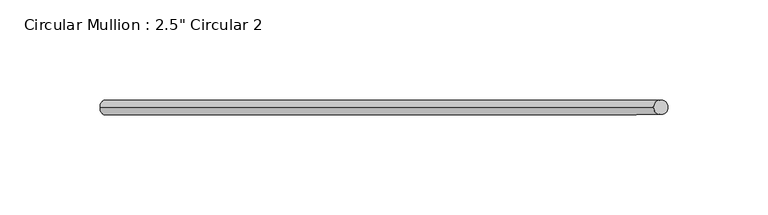
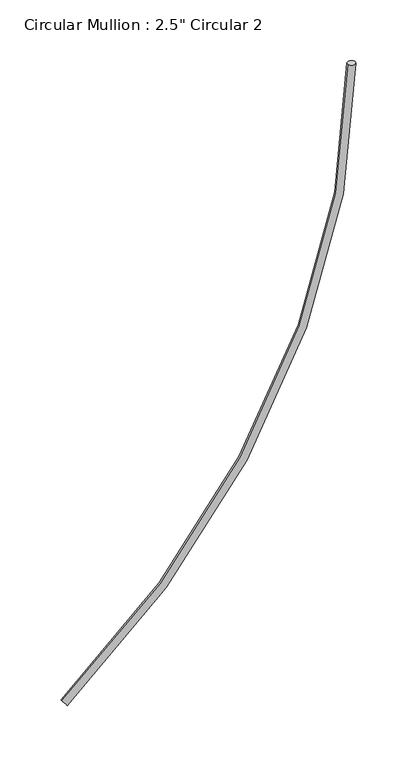
"""IFC4 building model written with IfcOpenShell, lengths in millimetres: member geometry."""

from ifc_helpers import new_model, si_unit, point, frame, origin, place, context, project, spatial, circle_curve, ellipse_curve, trimmed, source, transform, mapped, element, save
from ifc_brep_helpers import plane_surface, revolved_surface, advanced_brep


def member_43115751(model_context):
    return source(origin(), model_context, "Body", "AdvancedBrep", [
        advanced_brep(
        [(-283.7434, 0.0, -553.0088), (-7.239, 0.0, 0.0), (0.0, 0.0, 0.0), (-279.4, 0.0, -558.8)],
        [
            (0, 1, circle_curve(frame((-698.5, 0.0, 0.0), z_axis=(0.0, -1.0, 0.0), x_axis=(1.0, 0.0, 0.0)), 691.261)),
            (1, 2, circle_curve(frame((-3.6195, 0.0, 0.0), z_axis=(0.0, 0.0, -1.0), x_axis=(1.0, 0.0, 0.0)), 3.6195)),
            (2, 3, circle_curve(frame((-698.5, 0.0, 0.0), z_axis=(0.0, 1.0, 0.0), x_axis=(1.0, 0.0, 0.0)), 698.5)),
            (3, 0, circle_curve(frame((-281.5717, 0.0, -555.9044), z_axis=(0.8000000000000039, 0.0, 0.5999999999999948), x_axis=(0.5999999999999948, 0.0, -0.8000000000000039)), 3.6195)),
            (2, 1, circle_curve(frame((-3.6195, 0.0, 0.0), z_axis=(0.0, 0.0, -1.0), x_axis=(1.0, 0.0, 0.0)), 3.6195)),
            (0, 3, circle_curve(frame((-281.5717, 0.0, -555.9044), z_axis=(0.8000000000000039, 0.0, 0.5999999999999948), x_axis=(0.5999999999999948, 0.0, -0.8000000000000039)), 3.6195)),
        ],
        [
            revolved_surface(trimmed(ellipse_curve(frame((-3.6195, 0.0, 0.0), z_axis=(0.0, 0.0, 1.0), x_axis=(1.0, 0.0, 0.0)), 3.6195, 3.6195), [point((0.0, 0.0, 0.0))], [point((-7.239, 0.0, 0.0))], True, "CARTESIAN"), (-698.5, 0.0, 0.0), (0.0, 1.0, 0.0)),
            revolved_surface(trimmed(ellipse_curve(frame((-3.6195, 0.0, 0.0), z_axis=(0.0, 0.0, 1.0), x_axis=(1.0, 0.0, 0.0)), 3.6195, 3.6195), [point((-7.239, 0.0, 0.0))], [point((0.0, 0.0, 0.0))], True, "CARTESIAN"), (-698.5, 0.0, 0.0), (0.0, 1.0, 0.0)),
            plane_surface(frame((-304.8, 0.0, 0.0), z_axis=(0.0, 0.0, 1.0), x_axis=(0.0, 1.0, 0.0))),
            plane_surface(frame((-96.52, 0.0, -802.64), z_axis=(-0.800000000000004, 0.0, -0.5999999999999948), x_axis=(0.0, -1.0, 0.0))),
        ],
        [
            (0, [[1, 2, 3, 4]]),
            (1, [[-3, 5, -1, 6]]),
            (2, [[-2, -5]]),
            (3, [[-6, -4]]),
        ],
    ),
    ])


if __name__ == "__main__":
    model = new_model("IFC4")
    model_context = context("Model", 3, world=origin())
    ifc_project = project(units=[si_unit("LENGTHUNIT", "METRE", prefix="MILLI")], contexts=[model_context])
    site = spatial("IfcSite", under=ifc_project)
    building = spatial("IfcBuilding", under=site)
    placement = place(None, origin())
    member_shape = member_43115751(model_context)
    element("IfcMember", 1, ObjectType="Circular Mullion : 2.5\" Circular 2", at=placement, inside=building, context=model_context, shape_type="MappedRepresentation", body=[
        mapped(member_shape, transform((0.0, 0.0, 0.0), x_axis=(1.0, 0.0, 0.0), y_axis=(0.0, 1.0, 0.0), z_axis=(0.0, 0.0, 1.0))),
    ])
    save(model, "model.ifc")

# Revit data of these elements
# Type "Circular Mullion : 2.5\" Circular 2"
#   built-in parameter 1007350 = 0.011875 (stored number, unit not read)
# Element 1 (IfcMember, "Circular Mullion : 2.5\" Circular 2")
#   Materials on its faces: "Aluminum"
# Materials
#   "Aluminum": class "Metal", colour RGB 247 247 247, transparency 0, Description = "Aluminum 6061", Cost = 0
